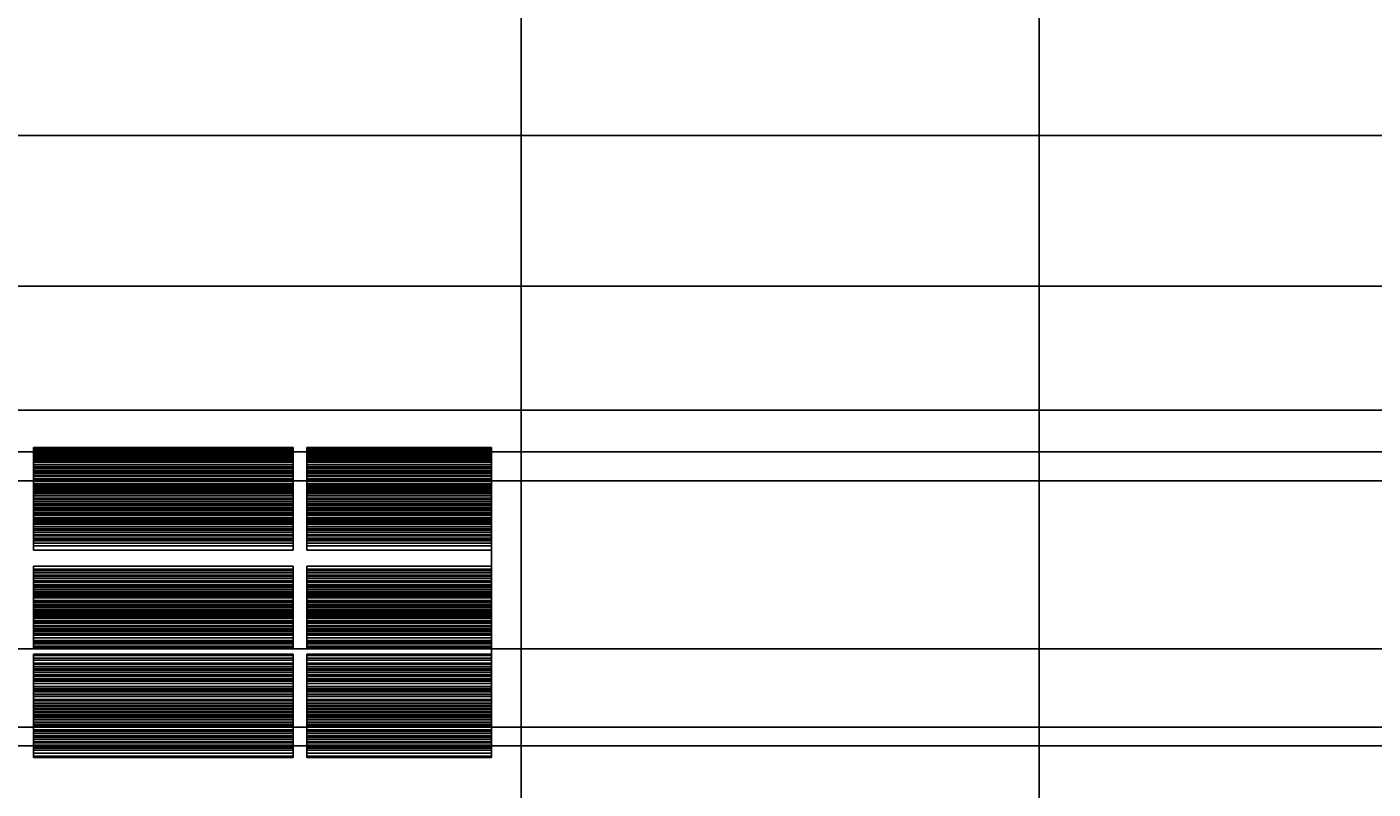
# Model space of a CAD drawing. Units: inches. Extents: x -32109 to 33221, y -19197 to 7608.
# Tile 22 of 25: x 15375 to 19011, y -59 to 1998. Entities that reach past the tile are written whole.
import ezdxf

# ---------------------------------------------------------------- set-up
doc = ezdxf.new("R2010")
doc.units = ezdxf.units.IN
doc.header["$MEASUREMENT"] = 0
doc.layers.add('A-ANNO-DIMS', color=2, linetype='Continuous', lineweight=18)
doc.layers.add('A-ELEV', color=7, linetype='Continuous', lineweight=25)
doc.styles.get("Standard").update_dxf_attribs({"font": 'arial.ttf'})
doc.dimstyles.get("Standard").update_dxf_attribs({"dimtxt": 0.18, "dimasz": 0.18, "dimexe": 0.18, "dimexo": 0.0625, "dimgap": 0.09, "dimtad": 0, "dimtih": 1, "dimtoh": 1, "dimdec": 4, "dimzin": 0, "dimdsep": 46, "dimtxsty": 'Standard', "dimcen": 0.09, "dimadec": 0, "dimazin": 0, "dimtfac": 1, "dimtdec": 4, "dimtofl": 0, "dimtmove": 0, "dimatfit": 3, "dimfxl": 1, "dimtolj": 1, "dimtzin": 0, "dimarcsym": 0})

# ---------------------------------------------------------------- blocks, each defined once
blk = doc.blocks.new('*D10')
at = {"layer": 'A-ANNO-DIMS', "color": 0, "lineweight": -2, "transparency": 16777216}
for p, q in [((-18512.6, -110.2), (-18512.6, 5772)), ((-18512.5, 5771.8), (-202.1, 5771.8)), ((18109.1, 5771.8), (-201.2, 5771.8)), ((18109.3, -101.5), (18109.3, 5772))]:
    blk.add_line(p, q, dxfattribs=at)
at = {"layer": 'A-ANNO-DIMS', "color": 0, "transparency": 16777216}
for points in [[(-18512.5, 5771.9), (-18512.5, 5771.8), (-18512.6, 5771.8)], [(18109.1, 5771.9), (18109.1, 5771.8), (18109.3, 5771.8)]]:
    blk.add_solid(points, dxfattribs=at)
at = {"layer": 'Defpoints', "color": 0, "transparency": 16777216}
for p in [(18109.3, 5771.8), (18109.3, -101.6), (-18512.6, -110.2)]:
    blk.add_point(p, dxfattribs=at)
at = {"layer": 'A-ANNO-DIMS', "color": 0, "transparency": 16777216, "insert": (-201.7, 5771.8), "char_height": 0.18, "attachment_point": 5}
blk.add_mtext('\\A1;36622', dxfattribs=at)
blk = doc.blocks.new('*D11')
at = {"layer": 'A-ANNO-DIMS', "color": 0, "lineweight": -2, "transparency": 16777216}
for p, q in [((14509.6, 1705.2), (25710.6, 1705.2)), ((25710.5, 1705), (25710.5, -209.6)), ((25710.5, -2124.6), (25710.5, -210)), ((-18512.6, -2124.8), (25710.6, -2124.8))]:
    blk.add_line(p, q, dxfattribs=at)
at = {"layer": 'A-ANNO-DIMS', "color": 0, "transparency": 16777216}
for points in [[(25710.4, 1705), (25710.5, 1705), (25710.5, 1705.2)], [(25710.4, -2124.6), (25710.5, -2124.6), (25710.5, -2124.8)]]:
    blk.add_solid(points, dxfattribs=at)
at = {"layer": 'Defpoints', "color": 0, "transparency": 16777216}
for p in [(14509.6, 1705.2), (-18512.6, -2124.8), (25710.5, -2124.8)]:
    blk.add_point(p, dxfattribs=at)
at = {"layer": 'A-ANNO-DIMS', "color": 0, "transparency": 16777216, "insert": (25710.5, -209.8), "char_height": 0.18, "attachment_point": 5}
blk.add_mtext('\\A1;3830', dxfattribs=at)
blk = doc.blocks.new('*D64')
at = {"layer": 'A-ANNO-DIMS', "color": 0, "lineweight": -2, "transparency": 16777216}
for p, q in [((14509.6, 1705.1), (14509.6, -5429.7)), ((15505.7, -101.7), (15505.7, -5429.7)), ((14509.7, -5429.6), (15007.3, -5429.6)), ((15505.6, -5429.6), (15008, -5429.6))]:
    blk.add_line(p, q, dxfattribs=at)
at = {"layer": 'A-ANNO-DIMS', "color": 0, "transparency": 16777216}
for points in [[(14509.7, -5429.5), (14509.7, -5429.6), (14509.6, -5429.6)], [(15505.6, -5429.5), (15505.6, -5429.6), (15505.7, -5429.6)]]:
    blk.add_solid(points, dxfattribs=at)
at = {"layer": 'Defpoints', "color": 0, "transparency": 16777216}
for p in [(14509.6, 1705.2), (15505.7, -101.6), (15505.7, -5429.6)]:
    blk.add_point(p, dxfattribs=at)
at = {"layer": 'A-ANNO-DIMS', "color": 0, "transparency": 16777216, "insert": (15007.6, -5429.6), "char_height": 0.18, "attachment_point": 5}
blk.add_mtext('\\A1;996.2', dxfattribs=at)
blk = doc.blocks.new('*D66')
at = {"layer": 'A-ANNO-DIMS', "color": 0, "lineweight": -2, "transparency": 16777216}
for p, q in [((14786.4, 963.8), (14786.4, 5772)), ((14786.6, 5771.8), (15747.7, 5771.8)), ((16709.6, 5771.8), (15748.6, 5771.8)), ((16709.8, 963.8), (16709.8, 5772))]:
    blk.add_line(p, q, dxfattribs=at)
at = {"layer": 'A-ANNO-DIMS', "color": 0, "transparency": 16777216}
for points in [[(14786.6, 5771.9), (14786.6, 5771.8), (14786.4, 5771.8)], [(16709.6, 5771.9), (16709.6, 5771.8), (16709.8, 5771.8)]]:
    blk.add_solid(points, dxfattribs=at)
at = {"layer": 'Defpoints', "color": 0, "transparency": 16777216}
for p in [(16709.8, 5771.8), (14786.4, 963.7), (16709.8, 963.7)]:
    blk.add_point(p, dxfattribs=at)
at = {"layer": 'A-ANNO-DIMS', "color": 0, "transparency": 16777216, "insert": (15748.1, 5771.8), "char_height": 0.18, "attachment_point": 5}
blk.add_mtext('\\A1;1923.4', dxfattribs=at)
blk = doc.blocks.new('*D67')
at = {"layer": 'A-ANNO-DIMS', "color": 0, "lineweight": -2, "transparency": 16777216}
for p, q in [((1645.9, 851.2), (25710.6, 851.2)), ((25710.5, 851), (25710.5, -632.3)), ((25710.5, -2116), (25710.5, -632.7)), ((1588.2, -2116.1), (25710.6, -2116.1))]:
    blk.add_line(p, q, dxfattribs=at)
at = {"layer": 'A-ANNO-DIMS', "color": 0, "transparency": 16777216}
for points in [[(25710.4, 851), (25710.5, 851), (25710.5, 851.2)], [(25710.4, -2116), (25710.5, -2116), (25710.5, -2116.1)]]:
    blk.add_solid(points, dxfattribs=at)
at = {"layer": 'Defpoints', "color": 0, "transparency": 16777216}
for p in [(1645.8, 851.2), (1588.2, -2116.1), (25710.5, -2116.1)]:
    blk.add_point(p, dxfattribs=at)
at = {"layer": 'A-ANNO-DIMS', "color": 0, "transparency": 16777216, "insert": (25710.5, -632.5), "char_height": 0.18, "attachment_point": 5}
blk.add_mtext('\\A1;2967.4', dxfattribs=at)
blk = doc.blocks.new('*D69')
at = {"layer": 'A-ANNO-DIMS', "color": 0, "lineweight": -2, "transparency": 16777216}
for p, q in [((5273.8, 1298.7), (25710.6, 1298.7)), ((25710.5, 1298.5), (25710.5, -411.9)), ((25710.5, -2122.6), (25710.5, -412.2)), ((5279.3, -2122.7), (25710.6, -2122.7))]:
    blk.add_line(p, q, dxfattribs=at)
at = {"layer": 'A-ANNO-DIMS', "color": 0, "transparency": 16777216}
for points in [[(25710.4, 1298.5), (25710.5, 1298.5), (25710.5, 1298.7)], [(25710.4, -2122.6), (25710.5, -2122.6), (25710.5, -2122.7)]]:
    blk.add_solid(points, dxfattribs=at)
at = {"layer": 'Defpoints', "color": 0, "transparency": 16777216}
for p in [(5273.7, 1298.7), (5279.3, -2122.7), (25710.5, -2122.7)]:
    blk.add_point(p, dxfattribs=at)
at = {"layer": 'A-ANNO-DIMS', "color": 0, "transparency": 16777216, "insert": (25710.5, -412), "char_height": 0.18, "attachment_point": 5}
blk.add_mtext('\\A1;3421.4', dxfattribs=at)
blk = doc.blocks.new('*D70')
at = {"layer": 'A-ANNO-DIMS', "color": 0, "lineweight": -2, "transparency": 16777216}
for p, q in [((8883.3, 57.8), (25710.6, 57.8)), ((25710.5, 57.6), (25710.5, -1045.1)), ((25710.5, -2148.2), (25710.5, -1045.5)), ((8832.4, -2148.4), (25710.6, -2148.4))]:
    blk.add_line(p, q, dxfattribs=at)
at = {"layer": 'A-ANNO-DIMS', "color": 0, "transparency": 16777216}
for points in [[(25710.4, 57.6), (25710.5, 57.6), (25710.5, 57.8)], [(25710.4, -2148.2), (25710.5, -2148.2), (25710.5, -2148.4)]]:
    blk.add_solid(points, dxfattribs=at)
at = {"layer": 'Defpoints', "color": 0, "transparency": 16777216}
for p in [(8883.2, 57.8), (8832.3, -2148.4), (25710.5, -2148.4)]:
    blk.add_point(p, dxfattribs=at)
at = {"layer": 'A-ANNO-DIMS', "color": 0, "transparency": 16777216, "insert": (25710.5, -1045.3), "char_height": 0.18, "attachment_point": 5}
blk.add_mtext('\\A1;2206', dxfattribs=at)
blk = doc.blocks.new('*D71')
at = {"layer": 'A-ANNO-DIMS', "color": 0, "lineweight": -2, "transparency": 16777216}
for p, q in [((11823.3, 772.8), (25710.6, 772.8)), ((25710.5, 772.6), (25710.5, 440.5)), ((25710.5, 107.9), (25710.5, 440.1)), ((11823.3, 107.7), (25710.6, 107.7))]:
    blk.add_line(p, q, dxfattribs=at)
at = {"layer": 'A-ANNO-DIMS', "color": 0, "transparency": 16777216}
for points in [[(25710.4, 772.6), (25710.5, 772.6), (25710.5, 772.8)], [(25710.4, 107.9), (25710.5, 107.9), (25710.5, 107.7)]]:
    blk.add_solid(points, dxfattribs=at)
at = {"layer": 'Defpoints', "color": 0, "transparency": 16777216}
for p in [(11823.2, 772.8), (11823.2, 107.7), (25710.5, 107.7)]:
    blk.add_point(p, dxfattribs=at)
at = {"layer": 'A-ANNO-DIMS', "color": 0, "transparency": 16777216, "insert": (25710.5, 440.3), "char_height": 0.18, "attachment_point": 5}
blk.add_mtext('\\A1;665.1', dxfattribs=at)
blk = doc.blocks.new('*D72')
at = {"layer": 'A-ANNO-DIMS', "color": 0, "lineweight": -2, "transparency": 16777216}
for p, q in [((11823.3, 107.7), (25710.6, 107.7)), ((25710.5, 107.6), (25710.5, -1004)), ((25710.5, -2116), (25710.5, -1004.4)), ((11383.7, -2116.1), (25710.6, -2116.1))]:
    blk.add_line(p, q, dxfattribs=at)
at = {"layer": 'A-ANNO-DIMS', "color": 0, "transparency": 16777216}
for points in [[(25710.4, 107.6), (25710.5, 107.6), (25710.5, 107.7)], [(25710.4, -2116), (25710.5, -2116), (25710.5, -2116.1)]]:
    blk.add_solid(points, dxfattribs=at)
at = {"layer": 'Defpoints', "color": 0, "transparency": 16777216}
for p in [(11823.2, 107.7), (11383.7, -2116.1), (25710.5, -2116.1)]:
    blk.add_point(p, dxfattribs=at)
at = {"layer": 'A-ANNO-DIMS', "color": 0, "transparency": 16777216, "insert": (25710.5, -1004.2), "char_height": 0.18, "attachment_point": 5}
blk.add_mtext('\\A1;2224', dxfattribs=at)
blk = doc.blocks.new('*D75')
at = {"layer": 'A-ANNO-DIMS', "color": 0, "lineweight": -2, "transparency": 16777216}
for p, q in [((14509.6, 1705.2), (25710.6, 1705.2)), ((25710.5, 1705), (25710.5, 1012.4)), ((25710.5, 319.4), (25710.5, 1012)), ((14509.6, 319.2), (25710.6, 319.2))]:
    blk.add_line(p, q, dxfattribs=at)
at = {"layer": 'A-ANNO-DIMS', "color": 0, "transparency": 16777216}
for points in [[(25710.4, 1705), (25710.5, 1705), (25710.5, 1705.2)], [(25710.4, 319.4), (25710.5, 319.4), (25710.5, 319.2)]]:
    blk.add_solid(points, dxfattribs=at)
at = {"layer": 'Defpoints', "color": 0, "transparency": 16777216}
for p in [(14509.6, 1705.2), (14509.6, 319.2), (25710.5, 319.2)]:
    blk.add_point(p, dxfattribs=at)
at = {"layer": 'A-ANNO-DIMS', "color": 0, "transparency": 16777216, "insert": (25710.5, 1012.2), "char_height": 0.18, "attachment_point": 5}
blk.add_mtext('\\A1;1386', dxfattribs=at)
blk = doc.blocks.new('*D76')
at = {"layer": 'A-ANNO-DIMS', "color": 0, "lineweight": -2, "transparency": 16777216}
for p, q in [((16709.9, 963.7), (25710.6, 963.7)), ((25710.5, 963.5), (25710.5, 431.2)), ((25710.5, -101.4), (25710.5, 430.9)), ((15505.8, -101.6), (25710.6, -101.6))]:
    blk.add_line(p, q, dxfattribs=at)
at = {"layer": 'A-ANNO-DIMS', "color": 0, "transparency": 16777216}
for points in [[(25710.4, 963.5), (25710.5, 963.5), (25710.5, 963.7)], [(25710.4, -101.4), (25710.5, -101.4), (25710.5, -101.6)]]:
    blk.add_solid(points, dxfattribs=at)
at = {"layer": 'Defpoints', "color": 0, "transparency": 16777216}
for p in [(16709.8, 963.7), (15505.7, -101.6), (25710.5, -101.6)]:
    blk.add_point(p, dxfattribs=at)
at = {"layer": 'A-ANNO-DIMS', "color": 0, "transparency": 16777216, "insert": (25710.5, 431.1), "char_height": 0.18, "attachment_point": 5}
blk.add_mtext('\\A1;1065.3', dxfattribs=at)

msp = doc.modelspace()

# ---------------------------------------------------------------- linework, layer by layer
at = {"layer": 'A-ELEV'}
for p, q in [((14786.396, 963.73), (16709.825, 963.73)), ((16709.825, 963.73), (16709.825, -101.6)), ((15393.197, 586.032), (15393.197, 862.63)), ((15393.197, 862.63), (16094.203, 862.63)), ((15393.197, 858.462), (16094.203, 858.462)), ((15393.197, 855.612), (16094.203, 855.612)), ((15393.197, 849.733), (16094.203, 849.733)), ((15393.197, 845.261), (16094.203, 845.261)), ((15393.197, 841.894), (16094.203, 841.894)), ((15393.197, 837.975), (16094.203, 837.975)), ((16094.203, 586.032), (16094.203, 862.63)), ((16130.611, 586.032), (16130.611, 862.63)), ((16130.611, 862.63), (16629.986, 862.63)), ((16130.611, 858.462), (16629.986, 858.462)), ((16130.611, 855.612), (16629.986, 855.612)), ((16130.611, 849.733), (16629.986, 849.733)), ((16130.611, 845.261), (16629.986, 845.261)), ((16130.611, 841.894), (16629.986, 841.894)), ((16130.611, 837.975), (16629.986, 837.975)), ((16629.986, 862.63), (16629.986, 25.622)), ((15393.197, 834.701), (16094.203, 834.701)), ((15393.197, 832.095), (16094.203, 832.095)), ((15393.197, 827.66), (16094.203, 827.66)), ((15393.197, 826.216), (16094.203, 826.216)), ((15393.197, 822.38), (16094.203, 822.38)), ((15393.197, 822.297), (16094.203, 822.297)), ((15393.197, 816.418), (16094.203, 816.418)), ((15393.197, 810.538), (16094.203, 810.538)), ((15393.197, 806.619), (16094.203, 806.619)), ((15393.197, 800.74), (16094.203, 800.74)), ((16130.611, 834.701), (16629.986, 834.701)), ((16130.611, 832.095), (16629.986, 832.095)), ((16130.611, 827.66), (16629.986, 827.66)), ((16130.611, 826.216), (16629.986, 826.216)), ((16130.611, 822.38), (16629.986, 822.38)), ((16130.611, 822.297), (16629.986, 822.297)), ((16130.611, 816.418), (16629.986, 816.418)), ((16130.611, 810.538), (16629.986, 810.538)), ((16130.611, 806.619), (16629.986, 806.619)), ((16130.611, 800.74), (16629.986, 800.74)), ((15393.197, 796.82), (16094.203, 796.82)), ((15393.197, 794.218), (16094.203, 794.218)), ((15393.197, 792.901), (16094.203, 792.901)), ((15393.197, 787.022), (16094.203, 787.022)), ((15393.197, 785.418), (16094.203, 785.418)), ((15393.197, 779.183), (16094.203, 779.183)), ((15393.197, 775.737), (16094.203, 775.737)), ((15393.197, 775.737), (16094.203, 775.737)), ((15393.197, 771.344), (16094.203, 771.344)), ((15393.197, 765.176), (16094.203, 765.176)), ((16130.611, 796.82), (16629.986, 796.82)), ((16130.611, 794.218), (16629.986, 794.218)), ((16130.611, 792.901), (16629.986, 792.901)), ((16130.611, 787.022), (16629.986, 787.022)), ((16130.611, 785.418), (16629.986, 785.418)), ((16130.611, 779.183), (16629.986, 779.183)), ((16130.611, 775.737), (16629.986, 775.737)), ((16130.611, 775.737), (16629.986, 775.737)), ((16130.611, 771.344), (16629.986, 771.344)), ((16130.611, 765.176), (16629.986, 765.176)), ((15393.197, 762.684), (16094.203, 762.684)), ((15393.197, 758.136), (16094.203, 758.136)), ((15393.197, 755.666), (16094.203, 755.666)), ((15393.197, 752.856), (16094.203, 752.856)), ((15393.197, 749.787), (16094.203, 749.787)), ((15393.197, 746.695), (16094.203, 746.695)), ((15393.197, 741.948), (16094.203, 741.948)), ((15393.197, 738.775), (16094.203, 738.775)), ((15393.197, 738.029), (16094.203, 738.029)), ((15393.197, 732.614), (16094.203, 732.614)), ((15393.197, 732.15), (16094.203, 732.15)), ((16130.611, 762.684), (16629.986, 762.684)), ((16130.611, 758.136), (16629.986, 758.136)), ((16130.611, 755.666), (16629.986, 755.666)), ((16130.611, 752.856), (16629.986, 752.856)), ((16130.611, 749.787), (16629.986, 749.787)), ((16130.611, 746.695), (16629.986, 746.695)), ((16130.611, 741.948), (16629.986, 741.948)), ((16130.611, 738.775), (16629.986, 738.775)), ((16130.611, 738.029), (16629.986, 738.029)), ((16130.611, 732.614), (16629.986, 732.614)), ((16130.611, 732.15), (16629.986, 732.15)), ((15393.197, 726.27), (16094.203, 726.27)), ((15393.197, 722.934), (16094.203, 722.934)), ((15393.197, 722.351), (16094.203, 722.351)), ((15393.197, 716.774), (16094.203, 716.774)), ((15393.197, 716.472), (16094.203, 716.472)), ((15393.197, 710.593), (16094.203, 710.593)), ((15393.197, 709.733), (16094.203, 709.733)), ((15393.197, 706.673), (16094.203, 706.673)), ((15393.197, 700.794), (16094.203, 700.794)), ((15393.197, 697.412), (16094.203, 697.412)), ((15393.197, 696.875), (16094.203, 696.875)), ((15393.197, 694.772), (16094.203, 694.772)), ((15393.197, 692.955), (16094.203, 692.955)), ((16130.611, 726.27), (16629.986, 726.27)), ((16130.611, 722.934), (16629.986, 722.934)), ((16130.611, 722.351), (16629.986, 722.351)), ((16130.611, 716.774), (16629.986, 716.774)), ((16130.611, 716.472), (16629.986, 716.472)), ((16130.611, 710.593), (16629.986, 710.593)), ((16130.611, 709.733), (16629.986, 709.733)), ((16130.611, 706.673), (16629.986, 706.673)), ((16130.611, 700.794), (16629.986, 700.794)), ((16130.611, 697.412), (16629.986, 697.412)), ((16130.611, 696.875), (16629.986, 696.875)), ((16130.611, 694.772), (16629.986, 694.772)), ((16130.611, 692.955), (16629.986, 692.955)), ((15393.197, 687.076), (16094.203, 687.076)), ((15393.197, 685.972), (16094.203, 685.972)), ((15393.197, 684.212), (16094.203, 684.212)), ((15393.197, 680.376), (16094.203, 680.376)), ((15393.197, 679.237), (16094.203, 679.237)), ((15393.197, 673.358), (16094.203, 673.358)), ((15393.197, 671.398), (16094.203, 671.398)), ((15393.197, 667.479), (16094.203, 667.479)), ((15393.197, 663.09), (16094.203, 663.09)), ((15393.197, 660.45), (16094.203, 660.45)), ((15393.197, 659.64), (16094.203, 659.64)), ((15393.197, 655.72), (16094.203, 655.72)), ((16130.611, 687.076), (16629.986, 687.076)), ((16130.611, 685.972), (16629.986, 685.972)), ((16130.611, 684.212), (16629.986, 684.212)), ((16130.611, 680.376), (16629.986, 680.376)), ((16130.611, 679.237), (16629.986, 679.237)), ((16130.611, 673.358), (16629.986, 673.358)), ((16130.611, 671.398), (16629.986, 671.398)), ((16130.611, 667.479), (16629.986, 667.479)), ((16130.611, 663.09), (16629.986, 663.09)), ((16130.611, 660.45), (16629.986, 660.45)), ((16130.611, 659.64), (16629.986, 659.64)), ((16130.611, 655.72), (16629.986, 655.72)), ((15393.197, 649.89), (16094.203, 649.89)), ((15393.197, 649.841), (16094.203, 649.841)), ((15393.197, 643.962), (16094.203, 643.962)), ((15393.197, 640.043), (16094.203, 640.043)), ((15393.197, 634.163), (16094.203, 634.163)), ((15393.197, 628.284), (16094.203, 628.284)), ((15393.197, 624.365), (16094.203, 624.365)), ((15393.197, 618.486), (16094.203, 618.486)), ((16130.611, 649.89), (16629.986, 649.89)), ((16130.611, 649.841), (16629.986, 649.841)), ((16130.611, 643.962), (16629.986, 643.962)), ((16130.611, 640.043), (16629.986, 640.043)), ((16130.611, 634.163), (16629.986, 634.163)), ((16130.611, 628.284), (16629.986, 628.284)), ((16130.611, 624.365), (16629.986, 624.365)), ((16130.611, 618.486), (16629.986, 618.486)), ((15393.197, 614.566), (16094.203, 614.566)), ((15393.197, 610.647), (16094.203, 610.647)), ((15393.197, 604.768), (16094.203, 604.768)), ((15393.197, 596.929), (16094.203, 596.929)), ((15393.197, 586.032), (16094.203, 586.032)), ((16130.611, 614.566), (16629.986, 614.566)), ((16130.611, 610.647), (16629.986, 610.647)), ((16130.611, 604.768), (16629.986, 604.768)), ((16130.611, 596.929), (16629.986, 596.929)), ((16130.611, 586.032), (16629.986, 586.032)), ((15393.197, 322.086), (15393.197, 542.056)), ((15393.197, 542.056), (16094.203, 542.056)), ((15393.197, 534.218), (16094.203, 534.218)), ((15393.197, 530.298), (16094.203, 530.298)), ((15393.197, 524.419), (16094.203, 524.419)), ((15393.197, 518.54), (16094.203, 518.54)), ((15393.197, 514.62), (16094.203, 514.62)), ((16094.203, 322.086), (16094.203, 542.056)), ((16130.611, 322.086), (16130.611, 542.056)), ((16130.611, 542.056), (16629.986, 542.056)), ((16130.611, 534.218), (16629.986, 534.218)), ((16130.611, 530.298), (16629.986, 530.298)), ((16130.611, 524.419), (16629.986, 524.419)), ((16130.611, 518.54), (16629.986, 518.54)), ((16130.611, 514.62), (16629.986, 514.62)), ((15393.197, 508.741), (16094.203, 508.741)), ((15393.197, 502.862), (16094.203, 502.862)), ((15393.197, 498.943), (16094.203, 498.943)), ((15393.197, 493.063), (16094.203, 493.063)), ((15393.197, 489.144), (16094.203, 489.144)), ((15393.197, 485.224), (16094.203, 485.224)), ((15393.197, 479.871), (16094.203, 479.871)), ((15393.197, 479.345), (16094.203, 479.345)), ((15393.197, 474.201), (16094.203, 474.201)), ((15393.197, 474.201), (16094.203, 474.201)), ((16130.611, 508.741), (16629.986, 508.741)), ((16130.611, 502.862), (16629.986, 502.862)), ((16130.611, 498.943), (16629.986, 498.943)), ((16130.611, 493.063), (16629.986, 493.063)), ((16130.611, 489.144), (16629.986, 489.144)), ((16130.611, 485.224), (16629.986, 485.224)), ((16130.611, 479.871), (16629.986, 479.871)), ((16130.611, 479.345), (16629.986, 479.345)), ((16130.611, 474.201), (16629.986, 474.201)), ((16130.611, 474.201), (16629.986, 474.201)), ((15393.197, 471.506), (16094.203, 471.506)), ((15393.197, 467.113), (16094.203, 467.113)), ((15393.197, 465.695), (16094.203, 465.695)), ((15393.197, 463.668), (16094.203, 463.668)), ((15393.197, 460.025), (16094.203, 460.025)), ((15393.197, 456.968), (16094.203, 456.968)), ((15393.197, 449.949), (16094.203, 449.949)), ((15393.197, 447.267), (16094.203, 447.267)), ((15393.197, 447.267), (16094.203, 447.267)), ((15393.197, 444.07), (16094.203, 444.07)), ((15393.197, 438.762), (16094.203, 438.762)), ((15393.197, 438.762), (16094.203, 438.762)), ((16130.611, 471.506), (16629.986, 471.506)), ((16130.611, 467.113), (16629.986, 467.113)), ((16130.611, 465.695), (16629.986, 465.695)), ((16130.611, 463.668), (16629.986, 463.668)), ((16130.611, 460.025), (16629.986, 460.025)), ((16130.611, 456.968), (16629.986, 456.968)), ((16130.611, 449.949), (16629.986, 449.949)), ((16130.611, 447.267), (16629.986, 447.267)), ((16130.611, 447.267), (16629.986, 447.267)), ((16130.611, 444.07), (16629.986, 444.07)), ((16130.611, 438.762), (16629.986, 438.762)), ((16130.611, 438.762), (16629.986, 438.762)), ((15393.197, 436.231), (16094.203, 436.231)), ((15393.197, 434.509), (16094.203, 434.509)), ((15393.197, 432.312), (16094.203, 432.312)), ((15393.197, 431.674), (16094.203, 431.674)), ((15393.197, 426.433), (16094.203, 426.433)), ((15393.197, 423.169), (16094.203, 423.169)), ((15393.197, 420.554), (16094.203, 420.554)), ((15393.197, 416.634), (16094.203, 416.634)), ((15393.197, 413.246), (16094.203, 413.246)), ((15393.197, 410.755), (16094.203, 410.755)), ((15393.197, 407.576), (16094.203, 407.576)), ((15393.197, 404.876), (16094.203, 404.876)), ((15393.197, 400.956), (16094.203, 400.956)), ((16130.611, 436.231), (16629.986, 436.231)), ((16130.611, 434.509), (16629.986, 434.509)), ((16130.611, 432.312), (16629.986, 432.312)), ((16130.611, 431.674), (16629.986, 431.674)), ((16130.611, 426.433), (16629.986, 426.433)), ((16130.611, 423.169), (16629.986, 423.169)), ((16130.611, 420.554), (16629.986, 420.554)), ((16130.611, 416.634), (16629.986, 416.634)), ((16130.611, 413.246), (16629.986, 413.246)), ((16130.611, 410.755), (16629.986, 410.755)), ((16130.611, 407.576), (16629.986, 407.576)), ((16130.611, 404.876), (16629.986, 404.876)), ((16130.611, 400.956), (16629.986, 400.956)), ((15393.197, 395.077), (16094.203, 395.077)), ((15393.197, 391.158), (16094.203, 391.158)), ((15393.197, 387.238), (16094.203, 387.238)), ((15393.197, 381.359), (16094.203, 381.359)), ((15393.197, 378.34), (16094.203, 378.34)), ((15393.197, 373.52), (16094.203, 373.52)), ((15393.197, 369.974), (16094.203, 369.974)), ((15393.197, 365.681), (16094.203, 365.681)), ((15393.197, 365.681), (16062.511, 365.681)), ((15393.197, 365.681), (16066.769, 365.681)), ((15393.197, 365.681), (16061.091, 365.681)), ((15393.197, 365.681), (16058.253, 365.681)), ((15393.197, 365.681), (16062.511, 365.681)), ((16130.611, 395.077), (16629.986, 395.077)), ((16130.611, 391.158), (16629.986, 391.158)), ((16130.611, 387.238), (16629.986, 387.238)), ((16130.611, 381.359), (16629.986, 381.359)), ((16130.611, 378.34), (16629.986, 378.34)), ((16130.611, 373.52), (16629.986, 373.52)), ((16130.611, 369.974), (16629.986, 369.974)), ((16130.611, 365.681), (16629.986, 365.681)), ((16130.611, 365.681), (16598.293, 365.681)), ((16130.611, 365.681), (16602.551, 365.681)), ((16130.611, 365.681), (16596.874, 365.681)), ((16130.611, 365.681), (16594.035, 365.681)), ((16130.611, 365.681), (16598.293, 365.681)), ((15393.197, 360.793), (16094.203, 360.793)), ((15393.197, 356.219), (16094.203, 356.219)), ((15393.197, 348.564), (16094.203, 348.564)), ((15393.197, 341.652), (16094.203, 341.652)), ((15393.197, 337.398), (16094.203, 337.398)), ((15393.197, 332.612), (16094.203, 332.612)), ((16130.611, 360.793), (16629.986, 360.793)), ((16130.611, 356.219), (16629.986, 356.219)), ((16130.611, 348.564), (16629.986, 348.564)), ((16130.611, 341.652), (16629.986, 341.652)), ((16130.611, 337.398), (16629.986, 337.398)), ((16130.611, 332.612), (16629.986, 332.612)), ((15393.197, 326.763), (16094.203, 326.763)), ((15393.197, 322.086), (16094.203, 322.086)), ((15393.197, 25.622), (15393.197, 305.269)), ((15393.197, 305.269), (16094.203, 305.269)), ((15393.197, 301.434), (16094.203, 301.434)), ((15393.197, 294.416), (16094.203, 294.416)), ((16094.203, 25.622), (16094.203, 305.269)), ((16130.611, 326.763), (16629.986, 326.763)), ((16130.611, 322.086), (16629.986, 322.086)), ((16130.611, 25.622), (16130.611, 305.269)), ((16130.611, 305.269), (16629.986, 305.269)), ((16130.611, 301.434), (16629.986, 301.434)), ((16130.611, 294.416), (16629.986, 294.416)), ((15393.197, 288.537), (16094.203, 288.537)), ((15393.197, 280.698), (16094.203, 280.698)), ((15393.197, 276.778), (16094.203, 276.778)), ((15393.197, 270.899), (16094.203, 270.899)), ((15393.197, 265.02), (16094.203, 265.02)), ((15393.197, 261.101), (16094.203, 261.101)), ((15393.197, 255.221), (16094.203, 255.221)), ((16130.611, 288.537), (16629.986, 288.537)), ((16130.611, 280.698), (16629.986, 280.698)), ((16130.611, 276.778), (16629.986, 276.778)), ((16130.611, 270.899), (16629.986, 270.899)), ((16130.611, 265.02), (16629.986, 265.02)), ((16130.611, 261.101), (16629.986, 261.101)), ((16130.611, 255.221), (16629.986, 255.221)), ((15393.197, 249.342), (16094.203, 249.342)), ((15393.197, 245.423), (16094.203, 245.423)), ((15393.197, 239.544), (16094.203, 239.544)), ((15393.197, 235.624), (16094.203, 235.624)), ((15393.197, 234.635), (16094.203, 234.635)), ((15393.197, 231.705), (16094.203, 231.705)), ((15393.197, 225.826), (16094.203, 225.826)), ((16130.611, 249.342), (16629.986, 249.342)), ((16130.611, 245.423), (16629.986, 245.423)), ((16130.611, 239.544), (16629.986, 239.544)), ((16130.611, 235.624), (16629.986, 235.624)), ((16130.611, 234.635), (16629.986, 234.635)), ((16130.611, 231.705), (16629.986, 231.705)), ((16130.611, 225.826), (16629.986, 225.826)), ((15393.197, 217.987), (16094.203, 217.987)), ((15393.197, 211.954), (16094.203, 211.954)), ((15393.197, 210.536), (16094.203, 210.536)), ((15393.197, 210.148), (16094.203, 210.148)), ((15393.197, 206.284), (16094.203, 206.284)), ((15393.197, 206.284), (16094.203, 206.284)), ((15393.197, 203.448), (16094.203, 203.448)), ((15393.197, 196.43), (16094.203, 196.43)), ((15393.197, 196.361), (16094.203, 196.361)), ((15393.197, 190.551), (16094.203, 190.551)), ((15393.197, 182.712), (16094.203, 182.712)), ((16130.611, 217.987), (16629.986, 217.987)), ((16130.611, 211.954), (16629.986, 211.954)), ((16130.611, 210.536), (16629.986, 210.536)), ((16130.611, 210.148), (16629.986, 210.148)), ((16130.611, 206.284), (16629.986, 206.284)), ((16130.611, 206.284), (16629.986, 206.284)), ((16130.611, 203.448), (16629.986, 203.448)), ((16130.611, 196.43), (16629.986, 196.43)), ((16130.611, 196.361), (16629.986, 196.361)), ((16130.611, 190.551), (16629.986, 190.551)), ((16130.611, 182.712), (16629.986, 182.712)), ((15393.197, 178.792), (16094.203, 178.792)), ((15393.197, 172.913), (16094.203, 172.913)), ((15393.197, 167.034), (16094.203, 167.034)), ((15393.197, 163.757), (16094.203, 163.757)), ((15393.197, 163.114), (16094.203, 163.114)), ((15393.197, 157.235), (16094.203, 157.235)), ((15393.197, 156.67), (16094.203, 156.67)), ((15393.197, 151.356), (16094.203, 151.356)), ((15393.197, 147.437), (16094.203, 147.437)), ((16130.611, 178.792), (16629.986, 178.792)), ((16130.611, 172.913), (16629.986, 172.913)), ((16130.611, 167.034), (16629.986, 167.034)), ((16130.611, 163.757), (16629.986, 163.757)), ((16130.611, 163.114), (16629.986, 163.114)), ((16130.611, 157.235), (16629.986, 157.235)), ((16130.611, 156.67), (16629.986, 156.67)), ((16130.611, 151.356), (16629.986, 151.356)), ((16130.611, 147.437), (16629.986, 147.437)), ((15393.197, 141.558), (16094.203, 141.558)), ((15393.197, 137.638), (16094.203, 137.638)), ((15393.197, 135.406), (16094.203, 135.406)), ((15393.197, 133.719), (16094.203, 133.719)), ((15393.197, 128.319), (16094.203, 128.319)), ((15393.197, 127.839), (16094.203, 127.839)), ((15393.197, 121.14), (16094.203, 121.14)), ((15393.197, 120.001), (16094.203, 120.001)), ((15393.197, 119.813), (16094.203, 119.813)), ((15393.197, 114.121), (16094.203, 114.121)), ((15393.197, 112.162), (16094.203, 112.162)), ((16130.611, 141.558), (16629.986, 141.558)), ((16130.611, 137.638), (16629.986, 137.638)), ((16130.611, 135.406), (16629.986, 135.406)), ((16130.611, 133.719), (16629.986, 133.719)), ((16130.611, 128.319), (16629.986, 128.319)), ((16130.611, 127.839), (16629.986, 127.839)), ((16130.611, 121.14), (16629.986, 121.14)), ((16130.611, 120.001), (16629.986, 120.001)), ((16130.611, 119.813), (16629.986, 119.813)), ((16130.611, 114.121), (16629.986, 114.121)), ((16130.611, 112.162), (16629.986, 112.162)), ((15393.197, 108.242), (16094.203, 108.242)), ((15393.197, 100.403), (16094.203, 100.403)), ((15393.197, 96.484), (16094.203, 96.484)), ((15393.197, 90.605), (16094.203, 90.605)), ((15393.197, 84.726), (16094.203, 84.726)), ((15393.197, 80.806), (16094.203, 80.806)), ((15393.197, 74.927), (16094.203, 74.927)), ((16130.611, 108.242), (16629.986, 108.242)), ((16130.611, 100.403), (16629.986, 100.403)), ((16130.611, 96.484), (16629.986, 96.484)), ((16130.611, 90.605), (16629.986, 90.605)), ((16130.611, 84.726), (16629.986, 84.726)), ((16130.611, 80.806), (16629.986, 80.806)), ((16130.611, 74.927), (16629.986, 74.927)), ((15393.197, 69.048), (16094.203, 69.048)), ((15393.197, 65.128), (16094.203, 65.128)), ((15393.197, 59.249), (16094.203, 59.249)), ((15393.197, 55.33), (16094.203, 55.33)), ((15393.197, 51.41), (16094.203, 51.41)), ((15393.197, 45.531), (16094.203, 45.531)), ((15393.197, 37.692), (16094.203, 37.692)), ((16130.611, 69.048), (16629.986, 69.048)), ((16130.611, 65.128), (16629.986, 65.128)), ((16130.611, 59.249), (16629.986, 59.249)), ((16130.611, 55.33), (16629.986, 55.33)), ((16130.611, 51.41), (16629.986, 51.41)), ((16130.611, 45.531), (16629.986, 45.531)), ((16130.611, 37.692), (16629.986, 37.692)), ((15393.197, 29.853), (16094.203, 29.853)), ((16094.203, 25.622), (15393.197, 25.622)), ((16130.611, 29.853), (16629.986, 29.853)), ((16629.986, 25.622), (16130.611, 25.622))]:
    msp.add_line(p, q, dxfattribs=at)

# ---------------------------------------------------------------- dimensions: what is measured, and where the dimension line sits
at = {"layer": 'A-ANNO-DIMS'}
for base, p1, p2, override, picture, middle in [((18109.317, 5771.835), (-18512.647, -110.242), (18109.317, -101.6), {"dimdec": 0, "dimlfac": 1, "dimrnd": 0, "dimzin": 0, "dimdsep": 46, "dimlunit": 2}, '*D10', (-201.665, 5771.835)), ((16709.825, 5771.835), (14786.396, 963.73), (16709.825, 963.73), {"dimdec": 1, "dimlfac": 1, "dimrnd": 0, "dimzin": 0, "dimdsep": 46, "dimlunit": 2}, '*D66', (15748.11, 5771.835)), ((15505.744, -5429.555), (14509.55, 1705.162), (15505.744, -101.6), {"dimdec": 1, "dimlfac": 1, "dimrnd": 0, "dimzin": 0, "dimdsep": 46, "dimlunit": 2}, '*D64', (15007.647, -5429.555))]:
    dim = msp.add_linear_dim(base=base, p1=p1, p2=p2, dimstyle='Standard', override=override, dxfattribs=at)
    dim.commit()
    dim.dimension.update_dxf_attribs({"geometry": picture, "text_midpoint": middle})
for base, p1, p2, override, picture, middle in [((25710.469, -2124.791), (14509.55, 1705.162), (-18512.647, -2124.791), {"dimdec": 0, "dimlfac": 1, "dimrnd": 0, "dimzin": 0, "dimdsep": 46, "dimlunit": 2}, '*D11', (25710.469, -209.814)), ((25710.469, 319.218), (14509.55, 1705.162), (14509.55, 319.218), {"dimdec": 0, "dimlfac": 1, "dimrnd": 0, "dimzin": 0, "dimdsep": 46, "dimlunit": 2}, '*D75', (25710.469, 1012.19)), ((25710.469, -2122.749), (5273.749, 1298.671), (5279.264, -2122.749), {"dimdec": 1, "dimlfac": 1, "dimrnd": 0, "dimzin": 0, "dimdsep": 46, "dimlunit": 2}, '*D69', (25710.469, -412.039)), ((25710.469, -101.6), (16709.825, 963.73), (15505.744, -101.6), {"dimdec": 1, "dimlfac": 1, "dimrnd": 0, "dimzin": 0, "dimdsep": 46, "dimlunit": 2}, '*D76', (25710.469, 431.065)), ((25710.469, -2116.149), (1645.845, 851.205), (1588.181, -2116.149), {"dimdec": 1, "dimlfac": 1, "dimrnd": 0, "dimzin": 0, "dimdsep": 46, "dimlunit": 2}, '*D67', (25710.469, -632.472)), ((25710.469, 107.745), (11823.239, 772.828), (11823.239, 107.745), {"dimdec": 1, "dimlfac": 1, "dimrnd": 0, "dimzin": 0, "dimdsep": 46, "dimlunit": 2}, '*D71', (25710.469, 440.287)), ((25710.469, -2116.149), (11823.239, 107.745), (11383.682, -2116.149), {"dimdec": 0, "dimlfac": 1, "dimrnd": 0, "dimzin": 0, "dimdsep": 46, "dimlunit": 2}, '*D72', (25710.469, -1004.202)), ((25710.469, -2148.367), (8883.215, 57.799), (8832.289, -2148.367), {"dimdec": 0, "dimlfac": 1, "dimrnd": 0, "dimzin": 0, "dimdsep": 46, "dimlunit": 2}, '*D70', (25710.469, -1045.284))]:
    dim = msp.add_linear_dim(base=base, p1=p1, p2=p2, angle=90, dimstyle='Standard', override=override, dxfattribs=at)
    dim.commit()
    dim.dimension.update_dxf_attribs({"geometry": picture, "text_midpoint": middle})

doc.saveas('drawing.dxf')
